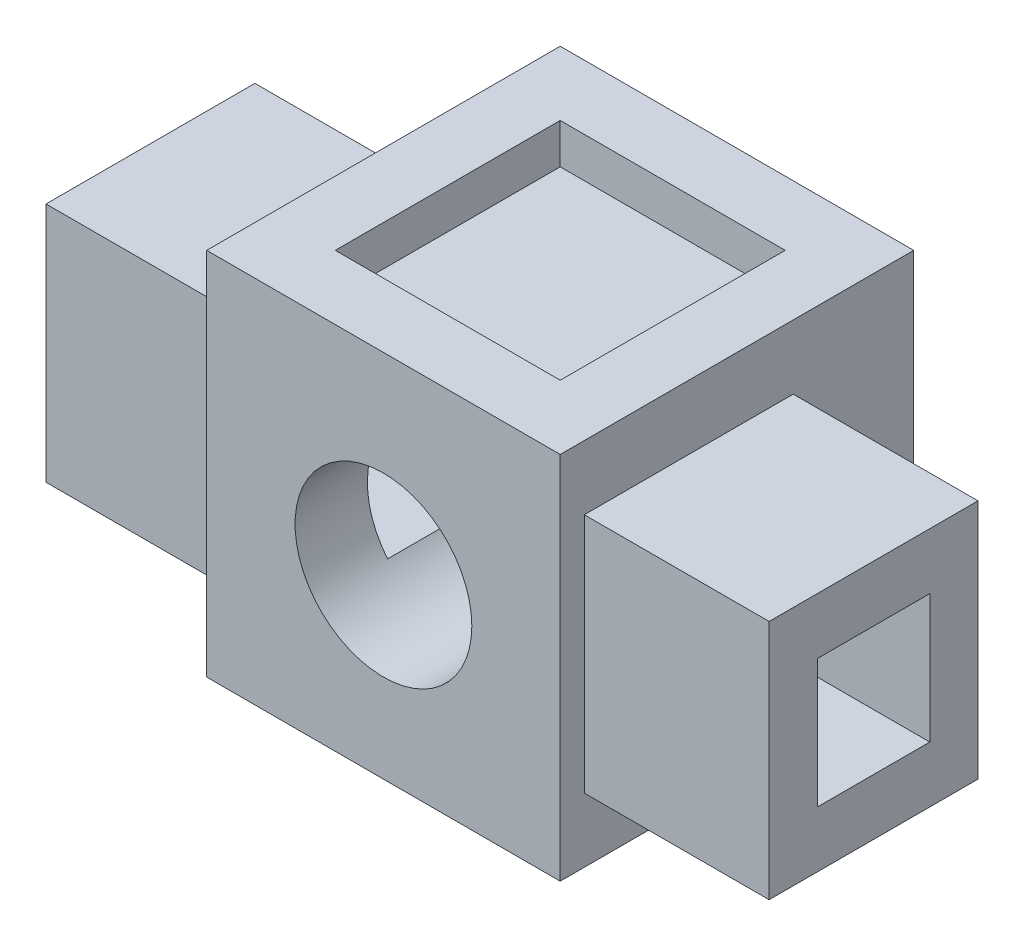
ISO-10303-21;
HEADER;
FILE_DESCRIPTION(('STEP AP214'),'2;1');
FILE_NAME('part.step','',(''),(''),'','','');
FILE_SCHEMA(('AUTOMOTIVE_DESIGN { 1 0 10303 214 1 1 1 1 }'));
ENDSEC;
DATA;
#1=APPLICATION_CONTEXT('core data for automotive mechanical design processes');
#2=APPLICATION_PROTOCOL_DEFINITION('international standard','automotive_design',2000,#1);
#3=PRODUCT_CONTEXT('',#1,'mechanical');
#4=PRODUCT('Part','Part','',(#3));
#5=PRODUCT_RELATED_PRODUCT_CATEGORY('part','',(#4));
#6=PRODUCT_DEFINITION_FORMATION('','',#4);
#7=PRODUCT_DEFINITION_CONTEXT('part definition',#1,'design');
#8=PRODUCT_DEFINITION('design','',#6,#7);
#9=PRODUCT_DEFINITION_SHAPE('','',#8);
#10=(LENGTH_UNIT() NAMED_UNIT(*) SI_UNIT(.MILLI.,.METRE.));
#11=(NAMED_UNIT(*) PLANE_ANGLE_UNIT() SI_UNIT($,.RADIAN.));
#12=(NAMED_UNIT(*) SI_UNIT($,.STERADIAN.) SOLID_ANGLE_UNIT());
#13=UNCERTAINTY_MEASURE_WITH_UNIT(LENGTH_MEASURE(1.E-05),#10,'distance_accuracy_value','');
#14=(GEOMETRIC_REPRESENTATION_CONTEXT(3) GLOBAL_UNCERTAINTY_ASSIGNED_CONTEXT((#13)) GLOBAL_UNIT_ASSIGNED_CONTEXT((#10,
#11,#12)) REPRESENTATION_CONTEXT('',''));
#15=CARTESIAN_POINT('',(0.,0.,0.));
#16=DIRECTION('',(0.,0.,1.));
#17=DIRECTION('',(1.,0.,0.));
#18=AXIS2_PLACEMENT_3D('',#15,#16,#17);
#19=CARTESIAN_POINT('',(22.,-23.,-44.));
#20=DIRECTION('',(1.,0.,0.));
#21=DIRECTION('',(0.,0.,-1.));
#22=AXIS2_PLACEMENT_3D('',#19,#20,#21);
#23=PLANE('',#22);
#24=DIRECTION('',(0.,1.,0.));
#25=VECTOR('',#24,1.);
#26=CARTESIAN_POINT('',(22.,-23.,0.));
#27=LINE('',#26,#25);
#28=CARTESIAN_POINT('',(22.,-23.,0.));
#29=VERTEX_POINT('',#28);
#30=CARTESIAN_POINT('',(22.,23.,0.));
#31=VERTEX_POINT('',#30);
#32=EDGE_CURVE('E360',#29,#31,#27,.T.);
#33=ORIENTED_EDGE('',*,*,#32,.F.);
#34=DIRECTION('',(0.,0.,1.));
#35=VECTOR('',#34,1.);
#36=CARTESIAN_POINT('',(22.,-23.,-44.));
#37=LINE('',#36,#35);
#38=CARTESIAN_POINT('',(22.,-23.,-44.));
#39=VERTEX_POINT('',#38);
#40=EDGE_CURVE('E11',#39,#29,#37,.T.);
#41=ORIENTED_EDGE('',*,*,#40,.F.);
#42=DIRECTION('',(0.,1.,0.));
#43=VECTOR('',#42,1.);
#44=CARTESIAN_POINT('',(22.,-23.,-44.));
#45=LINE('',#44,#43);
#46=CARTESIAN_POINT('',(22.,23.,-44.));
#47=VERTEX_POINT('',#46);
#48=EDGE_CURVE('E357',#39,#47,#45,.T.);
#49=ORIENTED_EDGE('',*,*,#48,.T.);
#50=DIRECTION('',(0.,0.,1.));
#51=VECTOR('',#50,1.);
#52=CARTESIAN_POINT('',(22.,23.,-44.));
#53=LINE('',#52,#51);
#54=EDGE_CURVE('E45',#47,#31,#53,.T.);
#55=ORIENTED_EDGE('',*,*,#54,.T.);
#56=EDGE_LOOP('',(#33,#41,#49,#55));
#57=FACE_BOUND('',#56,.T.);
#58=DIRECTION('',(0.,0.,1.));
#59=VECTOR('',#58,1.);
#60=CARTESIAN_POINT('',(22.,-15.,-29.));
#61=LINE('',#60,#59);
#62=CARTESIAN_POINT('',(22.,-15.,-29.));
#63=VERTEX_POINT('',#62);
#64=CARTESIAN_POINT('',(22.,-15.,-3.));
#65=VERTEX_POINT('',#64);
#66=EDGE_CURVE('E261',#63,#65,#61,.T.);
#67=ORIENTED_EDGE('',*,*,#66,.T.);
#68=DIRECTION('',(0.,1.,0.));
#69=VECTOR('',#68,1.);
#70=CARTESIAN_POINT('',(22.,15.,-3.));
#71=LINE('',#70,#69);
#72=CARTESIAN_POINT('',(22.,15.,-3.));
#73=VERTEX_POINT('',#72);
#74=EDGE_CURVE('E244',#65,#73,#71,.T.);
#75=ORIENTED_EDGE('',*,*,#74,.T.);
#76=DIRECTION('',(0.,0.,-1.));
#77=VECTOR('',#76,1.);
#78=CARTESIAN_POINT('',(22.,15.,-29.));
#79=LINE('',#78,#77);
#80=CARTESIAN_POINT('',(22.,15.,-29.));
#81=VERTEX_POINT('',#80);
#82=EDGE_CURVE('E249',#73,#81,#79,.T.);
#83=ORIENTED_EDGE('',*,*,#82,.T.);
#84=DIRECTION('',(0.,-1.,0.));
#85=VECTOR('',#84,1.);
#86=CARTESIAN_POINT('',(22.,15.,-29.));
#87=LINE('',#86,#85);
#88=EDGE_CURVE('E262',#81,#63,#87,.T.);
#89=ORIENTED_EDGE('',*,*,#88,.T.);
#90=EDGE_LOOP('',(#67,#75,#83,#89));
#91=FACE_BOUND('',#90,.T.);
#92=ADVANCED_FACE('F39',(#57,#91),#23,.T.);
#93=CARTESIAN_POINT('',(-22.,-23.,-44.));
#94=DIRECTION('',(-1.,0.,0.));
#95=DIRECTION('',(0.,0.,1.));
#96=AXIS2_PLACEMENT_3D('',#93,#94,#95);
#97=PLANE('',#96);
#98=DIRECTION('',(0.,-1.,0.));
#99=VECTOR('',#98,1.);
#100=CARTESIAN_POINT('',(-22.,-23.,0.));
#101=LINE('',#100,#99);
#102=CARTESIAN_POINT('',(-22.,23.,0.));
#103=VERTEX_POINT('',#102);
#104=CARTESIAN_POINT('',(-22.,-23.,0.));
#105=VERTEX_POINT('',#104);
#106=EDGE_CURVE('E378',#103,#105,#101,.T.);
#107=ORIENTED_EDGE('',*,*,#106,.F.);
#108=DIRECTION('',(0.,0.,1.));
#109=VECTOR('',#108,1.);
#110=CARTESIAN_POINT('',(-22.,23.,-44.));
#111=LINE('',#110,#109);
#112=CARTESIAN_POINT('',(-22.,23.,-44.));
#113=VERTEX_POINT('',#112);
#114=EDGE_CURVE('E382',#113,#103,#111,.T.);
#115=ORIENTED_EDGE('',*,*,#114,.F.);
#116=DIRECTION('',(0.,-1.,0.));
#117=VECTOR('',#116,1.);
#118=CARTESIAN_POINT('',(-22.,-23.,-44.));
#119=LINE('',#118,#117);
#120=CARTESIAN_POINT('',(-22.,-23.,-44.));
#121=VERTEX_POINT('',#120);
#122=EDGE_CURVE('E370',#113,#121,#119,.T.);
#123=ORIENTED_EDGE('',*,*,#122,.T.);
#124=DIRECTION('',(0.,0.,1.));
#125=VECTOR('',#124,1.);
#126=CARTESIAN_POINT('',(-22.,-23.,-44.));
#127=LINE('',#126,#125);
#128=EDGE_CURVE('E50',#121,#105,#127,.T.);
#129=ORIENTED_EDGE('',*,*,#128,.T.);
#130=EDGE_LOOP('',(#107,#115,#123,#129));
#131=FACE_BOUND('',#130,.T.);
#132=DIRECTION('',(0.,0.,-1.));
#133=VECTOR('',#132,1.);
#134=CARTESIAN_POINT('',(-22.,15.,-29.));
#135=LINE('',#134,#133);
#136=CARTESIAN_POINT('',(-22.,15.,-3.));
#137=VERTEX_POINT('',#136);
#138=CARTESIAN_POINT('',(-22.,15.,-29.));
#139=VERTEX_POINT('',#138);
#140=EDGE_CURVE('E308',#137,#139,#135,.T.);
#141=ORIENTED_EDGE('',*,*,#140,.F.);
#142=DIRECTION('',(0.,1.,0.));
#143=VECTOR('',#142,1.);
#144=CARTESIAN_POINT('',(-22.,15.,-3.));
#145=LINE('',#144,#143);
#146=CARTESIAN_POINT('',(-22.,-15.,-3.));
#147=VERTEX_POINT('',#146);
#148=EDGE_CURVE('E295',#147,#137,#145,.T.);
#149=ORIENTED_EDGE('',*,*,#148,.F.);
#150=DIRECTION('',(0.,0.,1.));
#151=VECTOR('',#150,1.);
#152=CARTESIAN_POINT('',(-22.,-15.,-29.));
#153=LINE('',#152,#151);
#154=CARTESIAN_POINT('',(-22.,-15.,-29.));
#155=VERTEX_POINT('',#154);
#156=EDGE_CURVE('E300',#155,#147,#153,.T.);
#157=ORIENTED_EDGE('',*,*,#156,.F.);
#158=DIRECTION('',(0.,-1.,0.));
#159=VECTOR('',#158,1.);
#160=CARTESIAN_POINT('',(-22.,15.,-29.));
#161=LINE('',#160,#159);
#162=EDGE_CURVE('E306',#139,#155,#161,.T.);
#163=ORIENTED_EDGE('',*,*,#162,.F.);
#164=EDGE_LOOP('',(#141,#149,#157,#163));
#165=FACE_BOUND('',#164,.T.);
#166=ADVANCED_FACE('F401',(#131,#165),#97,.T.);
#167=CARTESIAN_POINT('',(-22.,-23.,-44.));
#168=DIRECTION('',(0.,-1.,0.));
#169=DIRECTION('',(0.,0.,-1.));
#170=AXIS2_PLACEMENT_3D('',#167,#168,#169);
#171=PLANE('',#170);
#172=DIRECTION('',(1.,0.,0.));
#173=VECTOR('',#172,1.);
#174=CARTESIAN_POINT('',(-22.,-23.,0.));
#175=LINE('',#174,#173);
#176=EDGE_CURVE('E365',#105,#29,#175,.T.);
#177=ORIENTED_EDGE('',*,*,#176,.F.);
#178=ORIENTED_EDGE('',*,*,#128,.F.);
#179=DIRECTION('',(1.,0.,0.));
#180=VECTOR('',#179,1.);
#181=CARTESIAN_POINT('',(-22.,-23.,-44.));
#182=LINE('',#181,#180);
#183=EDGE_CURVE('E367',#121,#39,#182,.T.);
#184=ORIENTED_EDGE('',*,*,#183,.T.);
#185=ORIENTED_EDGE('',*,*,#40,.T.);
#186=EDGE_LOOP('',(#177,#178,#184,#185));
#187=FACE_BOUND('',#186,.T.);
#188=ADVANCED_FACE('F400',(#187),#171,.T.);
#189=CARTESIAN_POINT('',(-22.,23.,-44.));
#190=DIRECTION('',(0.,1.,0.));
#191=DIRECTION('',(0.,0.,1.));
#192=AXIS2_PLACEMENT_3D('',#189,#190,#191);
#193=PLANE('',#192);
#194=DIRECTION('',(0.,0.,-1.));
#195=VECTOR('',#194,1.);
#196=CARTESIAN_POINT('',(14.,23.,-8.));
#197=LINE('',#196,#195);
#198=CARTESIAN_POINT('',(14.,23.,-8.));
#199=VERTEX_POINT('',#198);
#200=CARTESIAN_POINT('',(14.,23.,-36.));
#201=VERTEX_POINT('',#200);
#202=EDGE_CURVE('E321',#199,#201,#197,.T.);
#203=ORIENTED_EDGE('',*,*,#202,.F.);
#204=DIRECTION('',(1.,0.,0.));
#205=VECTOR('',#204,1.);
#206=CARTESIAN_POINT('',(-14.,23.,-8.));
#207=LINE('',#206,#205);
#208=CARTESIAN_POINT('',(-14.,23.,-8.));
#209=VERTEX_POINT('',#208);
#210=EDGE_CURVE('E326',#209,#199,#207,.T.);
#211=ORIENTED_EDGE('',*,*,#210,.F.);
#212=DIRECTION('',(0.,0.,1.));
#213=VECTOR('',#212,1.);
#214=CARTESIAN_POINT('',(-14.,23.,-8.));
#215=LINE('',#214,#213);
#216=CARTESIAN_POINT('',(-14.,23.,-36.));
#217=VERTEX_POINT('',#216);
#218=EDGE_CURVE('E337',#217,#209,#215,.T.);
#219=ORIENTED_EDGE('',*,*,#218,.F.);
#220=DIRECTION('',(-1.,0.,0.));
#221=VECTOR('',#220,1.);
#222=CARTESIAN_POINT('',(-14.,23.,-36.));
#223=LINE('',#222,#221);
#224=EDGE_CURVE('E340',#201,#217,#223,.T.);
#225=ORIENTED_EDGE('',*,*,#224,.F.);
#226=EDGE_LOOP('',(#203,#211,#219,#225));
#227=FACE_BOUND('',#226,.T.);
#228=DIRECTION('',(-1.,0.,0.));
#229=VECTOR('',#228,1.);
#230=CARTESIAN_POINT('',(-22.,23.,0.));
#231=LINE('',#230,#229);
#232=EDGE_CURVE('E374',#31,#103,#231,.T.);
#233=ORIENTED_EDGE('',*,*,#232,.F.);
#234=ORIENTED_EDGE('',*,*,#54,.F.);
#235=DIRECTION('',(-1.,0.,0.));
#236=VECTOR('',#235,1.);
#237=CARTESIAN_POINT('',(-22.,23.,-44.));
#238=LINE('',#237,#236);
#239=EDGE_CURVE('E361',#47,#113,#238,.T.);
#240=ORIENTED_EDGE('',*,*,#239,.T.);
#241=ORIENTED_EDGE('',*,*,#114,.T.);
#242=EDGE_LOOP('',(#233,#234,#240,#241));
#243=FACE_BOUND('',#242,.T.);
#244=ADVANCED_FACE('F395',(#227,#243),#193,.T.);
#245=CARTESIAN_POINT('',(0.,0.,-44.));
#246=DIRECTION('',(0.,0.,-1.));
#247=DIRECTION('',(-1.,0.,0.));
#248=AXIS2_PLACEMENT_3D('',#245,#246,#247);
#249=PLANE('',#248);
#250=CARTESIAN_POINT('',(0.,-1.,-44.));
#251=DIRECTION('',(0.,0.,1.));
#252=DIRECTION('',(1.,0.,0.));
#253=AXIS2_PLACEMENT_3D('',#250,#251,#252);
#254=CIRCLE('',#253,11.);
#255=CARTESIAN_POINT('',(11.,-1.,-44.));
#256=VERTEX_POINT('',#255);
#257=EDGE_CURVE('E354',#256,#256,#254,.T.);
#258=ORIENTED_EDGE('',*,*,#257,.T.);
#259=EDGE_LOOP('',(#258));
#260=FACE_BOUND('',#259,.T.);
#261=ORIENTED_EDGE('',*,*,#48,.F.);
#262=ORIENTED_EDGE('',*,*,#183,.F.);
#263=ORIENTED_EDGE('',*,*,#122,.F.);
#264=ORIENTED_EDGE('',*,*,#239,.F.);
#265=EDGE_LOOP('',(#261,#262,#263,#264));
#266=FACE_BOUND('',#265,.T.);
#267=ADVANCED_FACE('F397',(#260,#266),#249,.T.);
#268=CARTESIAN_POINT('',(0.,0.,0.));
#269=DIRECTION('',(0.,0.,-1.));
#270=DIRECTION('',(-1.,0.,0.));
#271=AXIS2_PLACEMENT_3D('',#268,#269,#270);
#272=PLANE('',#271);
#273=CARTESIAN_POINT('',(0.,-1.,0.));
#274=DIRECTION('',(0.,0.,1.));
#275=DIRECTION('',(1.,0.,0.));
#276=AXIS2_PLACEMENT_3D('',#273,#274,#275);
#277=CIRCLE('',#276,11.);
#278=CARTESIAN_POINT('',(11.,-1.,0.));
#279=VERTEX_POINT('',#278);
#280=EDGE_CURVE('E350',#279,#279,#277,.T.);
#281=ORIENTED_EDGE('',*,*,#280,.F.);
#282=EDGE_LOOP('',(#281));
#283=FACE_BOUND('',#282,.T.);
#284=ORIENTED_EDGE('',*,*,#32,.T.);
#285=ORIENTED_EDGE('',*,*,#232,.T.);
#286=ORIENTED_EDGE('',*,*,#106,.T.);
#287=ORIENTED_EDGE('',*,*,#176,.T.);
#288=EDGE_LOOP('',(#284,#285,#286,#287));
#289=FACE_BOUND('',#288,.T.);
#290=ADVANCED_FACE('F394',(#283,#289),#272,.F.);
#291=CARTESIAN_POINT('',(0.,-1.,-44.));
#292=DIRECTION('',(0.,0.,1.));
#293=DIRECTION('',(1.,0.,0.));
#294=AXIS2_PLACEMENT_3D('',#291,#292,#293);
#295=CYLINDRICAL_SURFACE('',#294,11.);
#296=CARTESIAN_POINT('',(0.,-1.,-8.99999999999999));
#297=DIRECTION('',(0.,0.,1.));
#298=DIRECTION('',(0.,-1.,0.));
#299=AXIS2_PLACEMENT_3D('',#296,#297,#298);
#300=CIRCLE('',#299,11.);
#301=CARTESIAN_POINT('',(6.32455532033675,8.,-9.));
#302=VERTEX_POINT('',#301);
#303=CARTESIAN_POINT('',(8.48528137423857,-8.,-8.99999999999999));
#304=VERTEX_POINT('',#303);
#305=EDGE_CURVE('E224',#302,#304,#300,.F.);
#306=ORIENTED_EDGE('',*,*,#305,.T.);
#307=DIRECTION('',(0.,0.,1.));
#308=VECTOR('',#307,1.);
#309=CARTESIAN_POINT('',(8.48528137423857,-8.,-44.));
#310=LINE('',#309,#308);
#311=CARTESIAN_POINT('',(8.48528137423857,-8.,-23.));
#312=VERTEX_POINT('',#311);
#313=EDGE_CURVE('E202',#304,#312,#310,.F.);
#314=ORIENTED_EDGE('',*,*,#313,.T.);
#315=CARTESIAN_POINT('',(0.,-1.,-23.));
#316=DIRECTION('',(0.,0.,-1.));
#317=DIRECTION('',(-1.,0.,0.));
#318=AXIS2_PLACEMENT_3D('',#315,#316,#317);
#319=CIRCLE('',#318,11.);
#320=CARTESIAN_POINT('',(6.32455532033676,8.,-23.));
#321=VERTEX_POINT('',#320);
#322=EDGE_CURVE('E213',#312,#321,#319,.F.);
#323=ORIENTED_EDGE('',*,*,#322,.T.);
#324=DIRECTION('',(0.,0.,1.));
#325=VECTOR('',#324,1.);
#326=CARTESIAN_POINT('',(6.32455532033676,8.,-44.));
#327=LINE('',#326,#325);
#328=EDGE_CURVE('E220',#321,#302,#327,.T.);
#329=ORIENTED_EDGE('',*,*,#328,.T.);
#330=EDGE_LOOP('',(#306,#314,#323,#329));
#331=FACE_BOUND('',#330,.T.);
#332=CARTESIAN_POINT('',(-6.32455532033676,8.,-23.));
#333=VERTEX_POINT('',#332);
#334=CARTESIAN_POINT('',(-8.48528137423857,-8.,-23.));
#335=VERTEX_POINT('',#334);
#336=EDGE_CURVE('E217',#333,#335,#319,.F.);
#337=ORIENTED_EDGE('',*,*,#336,.T.);
#338=DIRECTION('',(0.,0.,1.));
#339=VECTOR('',#338,1.);
#340=CARTESIAN_POINT('',(-8.48528137423857,-8.,-44.));
#341=LINE('',#340,#339);
#342=CARTESIAN_POINT('',(-8.48528137423857,-8.,-8.99999999999999));
#343=VERTEX_POINT('',#342);
#344=EDGE_CURVE('E223',#335,#343,#341,.T.);
#345=ORIENTED_EDGE('',*,*,#344,.T.);
#346=CARTESIAN_POINT('',(-6.32455532033677,8.,-9.));
#347=VERTEX_POINT('',#346);
#348=EDGE_CURVE('E227',#343,#347,#300,.F.);
#349=ORIENTED_EDGE('',*,*,#348,.T.);
#350=DIRECTION('',(0.,0.,1.));
#351=VECTOR('',#350,1.);
#352=CARTESIAN_POINT('',(-6.32455532033676,8.,-44.));
#353=LINE('',#352,#351);
#354=EDGE_CURVE('E740',#347,#333,#353,.F.);
#355=ORIENTED_EDGE('',*,*,#354,.T.);
#356=EDGE_LOOP('',(#337,#345,#349,#355));
#357=FACE_BOUND('',#356,.T.);
#358=ORIENTED_EDGE('',*,*,#257,.F.);
#359=EDGE_LOOP('',(#358));
#360=FACE_BOUND('',#359,.T.);
#361=ORIENTED_EDGE('',*,*,#280,.T.);
#362=EDGE_LOOP('',(#361));
#363=FACE_BOUND('',#362,.T.);
#364=ADVANCED_FACE('F219',(#331,#357,#360,#363),#295,.F.);
#365=CARTESIAN_POINT('',(14.,18.,-8.));
#366=DIRECTION('',(1.,0.,0.));
#367=DIRECTION('',(0.,0.,-1.));
#368=AXIS2_PLACEMENT_3D('',#365,#366,#367);
#369=PLANE('',#368);
#370=ORIENTED_EDGE('',*,*,#202,.T.);
#371=DIRECTION('',(0.,1.,0.));
#372=VECTOR('',#371,1.);
#373=CARTESIAN_POINT('',(14.,18.,-36.));
#374=LINE('',#373,#372);
#375=CARTESIAN_POINT('',(14.,18.,-36.));
#376=VERTEX_POINT('',#375);
#377=EDGE_CURVE('E333',#376,#201,#374,.T.);
#378=ORIENTED_EDGE('',*,*,#377,.F.);
#379=DIRECTION('',(0.,0.,-1.));
#380=VECTOR('',#379,1.);
#381=CARTESIAN_POINT('',(14.,18.,-8.));
#382=LINE('',#381,#380);
#383=CARTESIAN_POINT('',(14.,18.,-8.));
#384=VERTEX_POINT('',#383);
#385=EDGE_CURVE('E325',#384,#376,#382,.T.);
#386=ORIENTED_EDGE('',*,*,#385,.F.);
#387=DIRECTION('',(0.,1.,0.));
#388=VECTOR('',#387,1.);
#389=CARTESIAN_POINT('',(14.,18.,-8.));
#390=LINE('',#389,#388);
#391=EDGE_CURVE('E342',#384,#199,#390,.T.);
#392=ORIENTED_EDGE('',*,*,#391,.T.);
#393=EDGE_LOOP('',(#370,#378,#386,#392));
#394=FACE_BOUND('',#393,.T.);
#395=ADVANCED_FACE('F499',(#394),#369,.F.);
#396=CARTESIAN_POINT('',(-14.,18.,-8.));
#397=DIRECTION('',(0.,0.,1.));
#398=DIRECTION('',(1.,0.,0.));
#399=AXIS2_PLACEMENT_3D('',#396,#397,#398);
#400=PLANE('',#399);
#401=ORIENTED_EDGE('',*,*,#210,.T.);
#402=ORIENTED_EDGE('',*,*,#391,.F.);
#403=DIRECTION('',(1.,0.,0.));
#404=VECTOR('',#403,1.);
#405=CARTESIAN_POINT('',(-14.,18.,-8.));
#406=LINE('',#405,#404);
#407=CARTESIAN_POINT('',(-14.,18.,-8.));
#408=VERTEX_POINT('',#407);
#409=EDGE_CURVE('E335',#408,#384,#406,.T.);
#410=ORIENTED_EDGE('',*,*,#409,.F.);
#411=DIRECTION('',(0.,1.,0.));
#412=VECTOR('',#411,1.);
#413=CARTESIAN_POINT('',(-14.,18.,-8.));
#414=LINE('',#413,#412);
#415=EDGE_CURVE('E346',#408,#209,#414,.T.);
#416=ORIENTED_EDGE('',*,*,#415,.T.);
#417=EDGE_LOOP('',(#401,#402,#410,#416));
#418=FACE_BOUND('',#417,.T.);
#419=ADVANCED_FACE('F602',(#418),#400,.F.);
#420=CARTESIAN_POINT('',(-14.,18.,-8.));
#421=DIRECTION('',(-1.,0.,0.));
#422=DIRECTION('',(0.,0.,1.));
#423=AXIS2_PLACEMENT_3D('',#420,#421,#422);
#424=PLANE('',#423);
#425=ORIENTED_EDGE('',*,*,#218,.T.);
#426=ORIENTED_EDGE('',*,*,#415,.F.);
#427=DIRECTION('',(0.,0.,1.));
#428=VECTOR('',#427,1.);
#429=CARTESIAN_POINT('',(-14.,18.,-8.));
#430=LINE('',#429,#428);
#431=CARTESIAN_POINT('',(-14.,18.,-36.));
#432=VERTEX_POINT('',#431);
#433=EDGE_CURVE('E328',#432,#408,#430,.T.);
#434=ORIENTED_EDGE('',*,*,#433,.F.);
#435=DIRECTION('',(0.,1.,0.));
#436=VECTOR('',#435,1.);
#437=CARTESIAN_POINT('',(-14.,18.,-36.));
#438=LINE('',#437,#436);
#439=EDGE_CURVE('E348',#432,#217,#438,.T.);
#440=ORIENTED_EDGE('',*,*,#439,.T.);
#441=EDGE_LOOP('',(#425,#426,#434,#440));
#442=FACE_BOUND('',#441,.T.);
#443=ADVANCED_FACE('F598',(#442),#424,.F.);
#444=CARTESIAN_POINT('',(-14.,18.,-36.));
#445=DIRECTION('',(0.,0.,-1.));
#446=DIRECTION('',(-1.,0.,0.));
#447=AXIS2_PLACEMENT_3D('',#444,#445,#446);
#448=PLANE('',#447);
#449=ORIENTED_EDGE('',*,*,#224,.T.);
#450=ORIENTED_EDGE('',*,*,#439,.F.);
#451=DIRECTION('',(-1.,0.,0.));
#452=VECTOR('',#451,1.);
#453=CARTESIAN_POINT('',(-14.,18.,-36.));
#454=LINE('',#453,#452);
#455=EDGE_CURVE('E324',#376,#432,#454,.T.);
#456=ORIENTED_EDGE('',*,*,#455,.F.);
#457=ORIENTED_EDGE('',*,*,#377,.T.);
#458=EDGE_LOOP('',(#449,#450,#456,#457));
#459=FACE_BOUND('',#458,.T.);
#460=ADVANCED_FACE('F595',(#459),#448,.F.);
#461=CARTESIAN_POINT('',(0.,18.,0.));
#462=DIRECTION('',(0.,-1.,0.));
#463=DIRECTION('',(0.,0.,-1.));
#464=AXIS2_PLACEMENT_3D('',#461,#462,#463);
#465=PLANE('',#464);
#466=ORIENTED_EDGE('',*,*,#385,.T.);
#467=ORIENTED_EDGE('',*,*,#455,.T.);
#468=ORIENTED_EDGE('',*,*,#433,.T.);
#469=ORIENTED_EDGE('',*,*,#409,.T.);
#470=EDGE_LOOP('',(#466,#467,#468,#469));
#471=FACE_BOUND('',#470,.T.);
#472=ADVANCED_FACE('F588',(#471),#465,.F.);
#473=CARTESIAN_POINT('',(-45.,0.,0.));
#474=DIRECTION('',(-1.,0.,0.));
#475=DIRECTION('',(0.,0.,1.));
#476=AXIS2_PLACEMENT_3D('',#473,#474,#475);
#477=PLANE('',#476);
#478=DIRECTION('',(0.,1.,0.));
#479=VECTOR('',#478,1.);
#480=CARTESIAN_POINT('',(-45.,15.,-3.));
#481=LINE('',#480,#479);
#482=CARTESIAN_POINT('',(-45.,-15.,-3.));
#483=VERTEX_POINT('',#482);
#484=CARTESIAN_POINT('',(-45.,15.,-3.));
#485=VERTEX_POINT('',#484);
#486=EDGE_CURVE('E291',#483,#485,#481,.T.);
#487=ORIENTED_EDGE('',*,*,#486,.T.);
#488=DIRECTION('',(0.,0.,-1.));
#489=VECTOR('',#488,1.);
#490=CARTESIAN_POINT('',(-45.,15.,-29.));
#491=LINE('',#490,#489);
#492=CARTESIAN_POINT('',(-45.,15.,-29.));
#493=VERTEX_POINT('',#492);
#494=EDGE_CURVE('E298',#485,#493,#491,.T.);
#495=ORIENTED_EDGE('',*,*,#494,.T.);
#496=DIRECTION('',(0.,-1.,0.));
#497=VECTOR('',#496,1.);
#498=CARTESIAN_POINT('',(-45.,15.,-29.));
#499=LINE('',#498,#497);
#500=CARTESIAN_POINT('',(-45.,-15.,-29.));
#501=VERTEX_POINT('',#500);
#502=EDGE_CURVE('E299',#493,#501,#499,.T.);
#503=ORIENTED_EDGE('',*,*,#502,.T.);
#504=DIRECTION('',(0.,0.,1.));
#505=VECTOR('',#504,1.);
#506=CARTESIAN_POINT('',(-45.,-15.,-29.));
#507=LINE('',#506,#505);
#508=EDGE_CURVE('E303',#501,#483,#507,.T.);
#509=ORIENTED_EDGE('',*,*,#508,.T.);
#510=EDGE_LOOP('',(#487,#495,#503,#509));
#511=FACE_BOUND('',#510,.T.);
#512=DIRECTION('',(0.,0.,-1.));
#513=VECTOR('',#512,1.);
#514=CARTESIAN_POINT('',(-45.,8.,-23.));
#515=LINE('',#514,#513);
#516=CARTESIAN_POINT('',(-45.,8.,-9.));
#517=VERTEX_POINT('',#516);
#518=CARTESIAN_POINT('',(-45.,8.,-23.));
#519=VERTEX_POINT('',#518);
#520=EDGE_CURVE('E276',#517,#519,#515,.T.);
#521=ORIENTED_EDGE('',*,*,#520,.F.);
#522=DIRECTION('',(0.,1.,0.));
#523=VECTOR('',#522,1.);
#524=CARTESIAN_POINT('',(-45.,8.,-9.));
#525=LINE('',#524,#523);
#526=CARTESIAN_POINT('',(-45.,-8.,-9.));
#527=VERTEX_POINT('',#526);
#528=EDGE_CURVE('E280',#527,#517,#525,.T.);
#529=ORIENTED_EDGE('',*,*,#528,.F.);
#530=DIRECTION('',(0.,0.,1.));
#531=VECTOR('',#530,1.);
#532=CARTESIAN_POINT('',(-45.,-8.,-23.));
#533=LINE('',#532,#531);
#534=CARTESIAN_POINT('',(-45.,-8.,-23.));
#535=VERTEX_POINT('',#534);
#536=EDGE_CURVE('E281',#535,#527,#533,.T.);
#537=ORIENTED_EDGE('',*,*,#536,.F.);
#538=DIRECTION('',(0.,-1.,0.));
#539=VECTOR('',#538,1.);
#540=CARTESIAN_POINT('',(-45.,8.,-23.));
#541=LINE('',#540,#539);
#542=EDGE_CURVE('E283',#519,#535,#541,.T.);
#543=ORIENTED_EDGE('',*,*,#542,.F.);
#544=EDGE_LOOP('',(#521,#529,#537,#543));
#545=FACE_BOUND('',#544,.T.);
#546=ADVANCED_FACE('F423',(#511,#545),#477,.T.);
#547=CARTESIAN_POINT('',(-45.,15.,-3.));
#548=DIRECTION('',(0.,0.,-1.));
#549=DIRECTION('',(0.,1.,0.));
#550=AXIS2_PLACEMENT_3D('',#547,#548,#549);
#551=PLANE('',#550);
#552=ORIENTED_EDGE('',*,*,#148,.T.);
#553=DIRECTION('',(1.,0.,0.));
#554=VECTOR('',#553,1.);
#555=CARTESIAN_POINT('',(-45.,15.,-3.));
#556=LINE('',#555,#554);
#557=EDGE_CURVE('E317',#485,#137,#556,.T.);
#558=ORIENTED_EDGE('',*,*,#557,.F.);
#559=ORIENTED_EDGE('',*,*,#486,.F.);
#560=DIRECTION('',(1.,0.,0.));
#561=VECTOR('',#560,1.);
#562=CARTESIAN_POINT('',(-45.,-15.,-3.));
#563=LINE('',#562,#561);
#564=EDGE_CURVE('E301',#483,#147,#563,.T.);
#565=ORIENTED_EDGE('',*,*,#564,.T.);
#566=EDGE_LOOP('',(#552,#558,#559,#565));
#567=FACE_BOUND('',#566,.T.);
#568=ADVANCED_FACE('F426',(#567),#551,.F.);
#569=CARTESIAN_POINT('',(-45.,15.,-29.));
#570=DIRECTION('',(0.,-1.,0.));
#571=DIRECTION('',(0.,0.,-1.));
#572=AXIS2_PLACEMENT_3D('',#569,#570,#571);
#573=PLANE('',#572);
#574=ORIENTED_EDGE('',*,*,#140,.T.);
#575=DIRECTION('',(1.,0.,0.));
#576=VECTOR('',#575,1.);
#577=CARTESIAN_POINT('',(-45.,15.,-29.));
#578=LINE('',#577,#576);
#579=EDGE_CURVE('E316',#493,#139,#578,.T.);
#580=ORIENTED_EDGE('',*,*,#579,.F.);
#581=ORIENTED_EDGE('',*,*,#494,.F.);
#582=ORIENTED_EDGE('',*,*,#557,.T.);
#583=EDGE_LOOP('',(#574,#580,#581,#582));
#584=FACE_BOUND('',#583,.T.);
#585=ADVANCED_FACE('F411',(#584),#573,.F.);
#586=CARTESIAN_POINT('',(-45.,15.,-29.));
#587=DIRECTION('',(0.,0.,1.));
#588=DIRECTION('',(0.,-1.,0.));
#589=AXIS2_PLACEMENT_3D('',#586,#587,#588);
#590=PLANE('',#589);
#591=ORIENTED_EDGE('',*,*,#162,.T.);
#592=DIRECTION('',(1.,0.,0.));
#593=VECTOR('',#592,1.);
#594=CARTESIAN_POINT('',(-45.,-15.,-29.));
#595=LINE('',#594,#593);
#596=EDGE_CURVE('E314',#501,#155,#595,.T.);
#597=ORIENTED_EDGE('',*,*,#596,.F.);
#598=ORIENTED_EDGE('',*,*,#502,.F.);
#599=ORIENTED_EDGE('',*,*,#579,.T.);
#600=EDGE_LOOP('',(#591,#597,#598,#599));
#601=FACE_BOUND('',#600,.T.);
#602=ADVANCED_FACE('F417',(#601),#590,.F.);
#603=CARTESIAN_POINT('',(-45.,-15.,-29.));
#604=DIRECTION('',(0.,1.,0.));
#605=DIRECTION('',(0.,0.,1.));
#606=AXIS2_PLACEMENT_3D('',#603,#604,#605);
#607=PLANE('',#606);
#608=ORIENTED_EDGE('',*,*,#156,.T.);
#609=ORIENTED_EDGE('',*,*,#564,.F.);
#610=ORIENTED_EDGE('',*,*,#508,.F.);
#611=ORIENTED_EDGE('',*,*,#596,.T.);
#612=EDGE_LOOP('',(#608,#609,#610,#611));
#613=FACE_BOUND('',#612,.T.);
#614=ADVANCED_FACE('F428',(#613),#607,.F.);
#615=CARTESIAN_POINT('',(-45.,8.,-9.));
#616=DIRECTION('',(0.,0.,-1.));
#617=DIRECTION('',(0.,1.,0.));
#618=AXIS2_PLACEMENT_3D('',#615,#616,#617);
#619=PLANE('',#618);
#620=DIRECTION('',(1.,0.,0.));
#621=VECTOR('',#620,1.);
#622=CARTESIAN_POINT('',(-45.,8.,-9.));
#623=LINE('',#622,#621);
#624=EDGE_CURVE('E287',#517,#347,#623,.T.);
#625=ORIENTED_EDGE('',*,*,#624,.T.);
#626=ORIENTED_EDGE('',*,*,#348,.F.);
#627=DIRECTION('',(1.,0.,0.));
#628=VECTOR('',#627,1.);
#629=CARTESIAN_POINT('',(-45.,-8.,-9.));
#630=LINE('',#629,#628);
#631=EDGE_CURVE('E282',#527,#343,#630,.T.);
#632=ORIENTED_EDGE('',*,*,#631,.F.);
#633=ORIENTED_EDGE('',*,*,#528,.T.);
#634=EDGE_LOOP('',(#625,#626,#632,#633));
#635=FACE_BOUND('',#634,.T.);
#636=ADVANCED_FACE('F429',(#635),#619,.T.);
#637=CARTESIAN_POINT('',(-45.,8.,-23.));
#638=DIRECTION('',(0.,-1.,0.));
#639=DIRECTION('',(0.,0.,-1.));
#640=AXIS2_PLACEMENT_3D('',#637,#638,#639);
#641=PLANE('',#640);
#642=DIRECTION('',(1.,0.,0.));
#643=VECTOR('',#642,1.);
#644=CARTESIAN_POINT('',(-45.,8.,-23.));
#645=LINE('',#644,#643);
#646=EDGE_CURVE('E286',#519,#333,#645,.T.);
#647=ORIENTED_EDGE('',*,*,#646,.T.);
#648=ORIENTED_EDGE('',*,*,#354,.F.);
#649=ORIENTED_EDGE('',*,*,#624,.F.);
#650=ORIENTED_EDGE('',*,*,#520,.T.);
#651=EDGE_LOOP('',(#647,#648,#649,#650));
#652=FACE_BOUND('',#651,.T.);
#653=ADVANCED_FACE('F440',(#652),#641,.T.);
#654=CARTESIAN_POINT('',(-45.,8.,-23.));
#655=DIRECTION('',(0.,0.,1.));
#656=DIRECTION('',(1.,0.,0.));
#657=AXIS2_PLACEMENT_3D('',#654,#655,#656);
#658=PLANE('',#657);
#659=DIRECTION('',(1.,0.,0.));
#660=VECTOR('',#659,1.);
#661=CARTESIAN_POINT('',(-45.,-8.,-23.));
#662=LINE('',#661,#660);
#663=EDGE_CURVE('E61',#535,#335,#662,.T.);
#664=ORIENTED_EDGE('',*,*,#663,.T.);
#665=ORIENTED_EDGE('',*,*,#336,.F.);
#666=ORIENTED_EDGE('',*,*,#646,.F.);
#667=ORIENTED_EDGE('',*,*,#542,.T.);
#668=EDGE_LOOP('',(#664,#665,#666,#667));
#669=FACE_BOUND('',#668,.T.);
#670=ADVANCED_FACE('F513',(#669),#658,.T.);
#671=CARTESIAN_POINT('',(-45.,-8.,-23.));
#672=DIRECTION('',(0.,1.,0.));
#673=DIRECTION('',(0.,0.,1.));
#674=AXIS2_PLACEMENT_3D('',#671,#672,#673);
#675=PLANE('',#674);
#676=ORIENTED_EDGE('',*,*,#631,.T.);
#677=ORIENTED_EDGE('',*,*,#344,.F.);
#678=ORIENTED_EDGE('',*,*,#663,.F.);
#679=ORIENTED_EDGE('',*,*,#536,.T.);
#680=EDGE_LOOP('',(#676,#677,#678,#679));
#681=FACE_BOUND('',#680,.T.);
#682=ADVANCED_FACE('F454',(#681),#675,.T.);
#683=CARTESIAN_POINT('',(45.,15.,-3.));
#684=DIRECTION('',(0.,0.,1.));
#685=DIRECTION('',(0.,-1.,0.));
#686=AXIS2_PLACEMENT_3D('',#683,#684,#685);
#687=PLANE('',#686);
#688=ORIENTED_EDGE('',*,*,#74,.F.);
#689=DIRECTION('',(-1.,0.,0.));
#690=VECTOR('',#689,1.);
#691=CARTESIAN_POINT('',(45.,-15.,-3.));
#692=LINE('',#691,#690);
#693=CARTESIAN_POINT('',(45.,-15.,-3.));
#694=VERTEX_POINT('',#693);
#695=EDGE_CURVE('E273',#694,#65,#692,.T.);
#696=ORIENTED_EDGE('',*,*,#695,.F.);
#697=DIRECTION('',(0.,1.,0.));
#698=VECTOR('',#697,1.);
#699=CARTESIAN_POINT('',(45.,15.,-3.));
#700=LINE('',#699,#698);
#701=CARTESIAN_POINT('',(45.,15.,-3.));
#702=VERTEX_POINT('',#701);
#703=EDGE_CURVE('E242',#694,#702,#700,.T.);
#704=ORIENTED_EDGE('',*,*,#703,.T.);
#705=DIRECTION('',(-1.,0.,0.));
#706=VECTOR('',#705,1.);
#707=CARTESIAN_POINT('',(45.,15.,-3.));
#708=LINE('',#707,#706);
#709=EDGE_CURVE('E256',#702,#73,#708,.T.);
#710=ORIENTED_EDGE('',*,*,#709,.T.);
#711=EDGE_LOOP('',(#688,#696,#704,#710));
#712=FACE_BOUND('',#711,.T.);
#713=ADVANCED_FACE('F449',(#712),#687,.T.);
#714=CARTESIAN_POINT('',(45.,-15.,-29.));
#715=DIRECTION('',(0.,-1.,0.));
#716=DIRECTION('',(0.,0.,-1.));
#717=AXIS2_PLACEMENT_3D('',#714,#715,#716);
#718=PLANE('',#717);
#719=ORIENTED_EDGE('',*,*,#66,.F.);
#720=DIRECTION('',(-1.,0.,0.));
#721=VECTOR('',#720,1.);
#722=CARTESIAN_POINT('',(45.,-15.,-29.));
#723=LINE('',#722,#721);
#724=CARTESIAN_POINT('',(45.,-15.,-29.));
#725=VERTEX_POINT('',#724);
#726=EDGE_CURVE('E275',#725,#63,#723,.T.);
#727=ORIENTED_EDGE('',*,*,#726,.F.);
#728=DIRECTION('',(0.,0.,1.));
#729=VECTOR('',#728,1.);
#730=CARTESIAN_POINT('',(45.,-15.,-29.));
#731=LINE('',#730,#729);
#732=EDGE_CURVE('E246',#725,#694,#731,.T.);
#733=ORIENTED_EDGE('',*,*,#732,.T.);
#734=ORIENTED_EDGE('',*,*,#695,.T.);
#735=EDGE_LOOP('',(#719,#727,#733,#734));
#736=FACE_BOUND('',#735,.T.);
#737=ADVANCED_FACE('F451',(#736),#718,.T.);
#738=CARTESIAN_POINT('',(45.,15.,-29.));
#739=DIRECTION('',(0.,0.,-1.));
#740=DIRECTION('',(0.,1.,0.));
#741=AXIS2_PLACEMENT_3D('',#738,#739,#740);
#742=PLANE('',#741);
#743=ORIENTED_EDGE('',*,*,#88,.F.);
#744=DIRECTION('',(-1.,0.,0.));
#745=VECTOR('',#744,1.);
#746=CARTESIAN_POINT('',(45.,15.,-29.));
#747=LINE('',#746,#745);
#748=CARTESIAN_POINT('',(45.,15.,-29.));
#749=VERTEX_POINT('',#748);
#750=EDGE_CURVE('E269',#749,#81,#747,.T.);
#751=ORIENTED_EDGE('',*,*,#750,.F.);
#752=DIRECTION('',(0.,-1.,0.));
#753=VECTOR('',#752,1.);
#754=CARTESIAN_POINT('',(45.,15.,-29.));
#755=LINE('',#754,#753);
#756=EDGE_CURVE('E252',#749,#725,#755,.T.);
#757=ORIENTED_EDGE('',*,*,#756,.T.);
#758=ORIENTED_EDGE('',*,*,#726,.T.);
#759=EDGE_LOOP('',(#743,#751,#757,#758));
#760=FACE_BOUND('',#759,.T.);
#761=ADVANCED_FACE('F465',(#760),#742,.T.);
#762=CARTESIAN_POINT('',(45.,15.,-29.));
#763=DIRECTION('',(0.,1.,0.));
#764=DIRECTION('',(0.,0.,1.));
#765=AXIS2_PLACEMENT_3D('',#762,#763,#764);
#766=PLANE('',#765);
#767=ORIENTED_EDGE('',*,*,#82,.F.);
#768=ORIENTED_EDGE('',*,*,#709,.F.);
#769=DIRECTION('',(0.,0.,-1.));
#770=VECTOR('',#769,1.);
#771=CARTESIAN_POINT('',(45.,15.,-29.));
#772=LINE('',#771,#770);
#773=EDGE_CURVE('E254',#702,#749,#772,.T.);
#774=ORIENTED_EDGE('',*,*,#773,.T.);
#775=ORIENTED_EDGE('',*,*,#750,.T.);
#776=EDGE_LOOP('',(#767,#768,#774,#775));
#777=FACE_BOUND('',#776,.T.);
#778=ADVANCED_FACE('F473',(#777),#766,.T.);
#779=CARTESIAN_POINT('',(45.,0.,0.));
#780=DIRECTION('',(1.,0.,0.));
#781=DIRECTION('',(0.,0.,1.));
#782=AXIS2_PLACEMENT_3D('',#779,#780,#781);
#783=PLANE('',#782);
#784=DIRECTION('',(0.,1.,0.));
#785=VECTOR('',#784,1.);
#786=CARTESIAN_POINT('',(45.,8.,-9.));
#787=LINE('',#786,#785);
#788=CARTESIAN_POINT('',(45.,-8.,-9.));
#789=VERTEX_POINT('',#788);
#790=CARTESIAN_POINT('',(45.,8.,-9.));
#791=VERTEX_POINT('',#790);
#792=EDGE_CURVE('E221',#789,#791,#787,.T.);
#793=ORIENTED_EDGE('',*,*,#792,.T.);
#794=DIRECTION('',(0.,0.,-1.));
#795=VECTOR('',#794,1.);
#796=CARTESIAN_POINT('',(45.,8.,-23.));
#797=LINE('',#796,#795);
#798=CARTESIAN_POINT('',(45.,8.,-23.));
#799=VERTEX_POINT('',#798);
#800=EDGE_CURVE('E240',#791,#799,#797,.T.);
#801=ORIENTED_EDGE('',*,*,#800,.T.);
#802=DIRECTION('',(0.,-1.,0.));
#803=VECTOR('',#802,1.);
#804=CARTESIAN_POINT('',(45.,8.,-23.));
#805=LINE('',#804,#803);
#806=CARTESIAN_POINT('',(45.,-8.,-23.));
#807=VERTEX_POINT('',#806);
#808=EDGE_CURVE('E232',#799,#807,#805,.T.);
#809=ORIENTED_EDGE('',*,*,#808,.T.);
#810=DIRECTION('',(0.,0.,1.));
#811=VECTOR('',#810,1.);
#812=CARTESIAN_POINT('',(45.,-8.,-23.));
#813=LINE('',#812,#811);
#814=EDGE_CURVE('E208',#807,#789,#813,.T.);
#815=ORIENTED_EDGE('',*,*,#814,.T.);
#816=EDGE_LOOP('',(#793,#801,#809,#815));
#817=FACE_BOUND('',#816,.T.);
#818=ORIENTED_EDGE('',*,*,#703,.F.);
#819=ORIENTED_EDGE('',*,*,#732,.F.);
#820=ORIENTED_EDGE('',*,*,#756,.F.);
#821=ORIENTED_EDGE('',*,*,#773,.F.);
#822=EDGE_LOOP('',(#818,#819,#820,#821));
#823=FACE_BOUND('',#822,.T.);
#824=ADVANCED_FACE('F477',(#817,#823),#783,.T.);
#825=CARTESIAN_POINT('',(45.,8.,-9.));
#826=DIRECTION('',(0.,0.,1.));
#827=DIRECTION('',(0.,-1.,0.));
#828=AXIS2_PLACEMENT_3D('',#825,#826,#827);
#829=PLANE('',#828);
#830=DIRECTION('',(-1.,0.,0.));
#831=VECTOR('',#830,1.);
#832=CARTESIAN_POINT('',(45.,-8.,-9.));
#833=LINE('',#832,#831);
#834=EDGE_CURVE('E209',#789,#304,#833,.T.);
#835=ORIENTED_EDGE('',*,*,#834,.T.);
#836=ORIENTED_EDGE('',*,*,#305,.F.);
#837=DIRECTION('',(-1.,0.,0.));
#838=VECTOR('',#837,1.);
#839=CARTESIAN_POINT('',(45.,8.,-9.));
#840=LINE('',#839,#838);
#841=EDGE_CURVE('E238',#791,#302,#840,.T.);
#842=ORIENTED_EDGE('',*,*,#841,.F.);
#843=ORIENTED_EDGE('',*,*,#792,.F.);
#844=EDGE_LOOP('',(#835,#836,#842,#843));
#845=FACE_BOUND('',#844,.T.);
#846=ADVANCED_FACE('F487',(#845),#829,.F.);
#847=CARTESIAN_POINT('',(45.,-8.,-23.));
#848=DIRECTION('',(0.,-1.,0.));
#849=DIRECTION('',(0.,0.,-1.));
#850=AXIS2_PLACEMENT_3D('',#847,#848,#849);
#851=PLANE('',#850);
#852=DIRECTION('',(-1.,0.,0.));
#853=VECTOR('',#852,1.);
#854=CARTESIAN_POINT('',(45.,-8.,-23.));
#855=LINE('',#854,#853);
#856=EDGE_CURVE('E205',#807,#312,#855,.T.);
#857=ORIENTED_EDGE('',*,*,#856,.T.);
#858=ORIENTED_EDGE('',*,*,#313,.F.);
#859=ORIENTED_EDGE('',*,*,#834,.F.);
#860=ORIENTED_EDGE('',*,*,#814,.F.);
#861=EDGE_LOOP('',(#857,#858,#859,#860));
#862=FACE_BOUND('',#861,.T.);
#863=ADVANCED_FACE('F201',(#862),#851,.F.);
#864=CARTESIAN_POINT('',(45.,8.,-23.));
#865=DIRECTION('',(0.,0.,-1.));
#866=DIRECTION('',(-1.,0.,0.));
#867=AXIS2_PLACEMENT_3D('',#864,#865,#866);
#868=PLANE('',#867);
#869=DIRECTION('',(-1.,0.,0.));
#870=VECTOR('',#869,1.);
#871=CARTESIAN_POINT('',(45.,8.,-23.));
#872=LINE('',#871,#870);
#873=EDGE_CURVE('E54',#799,#321,#872,.T.);
#874=ORIENTED_EDGE('',*,*,#873,.T.);
#875=ORIENTED_EDGE('',*,*,#322,.F.);
#876=ORIENTED_EDGE('',*,*,#856,.F.);
#877=ORIENTED_EDGE('',*,*,#808,.F.);
#878=EDGE_LOOP('',(#874,#875,#876,#877));
#879=FACE_BOUND('',#878,.T.);
#880=ADVANCED_FACE('F212',(#879),#868,.F.);
#881=CARTESIAN_POINT('',(45.,8.,-23.));
#882=DIRECTION('',(0.,1.,0.));
#883=DIRECTION('',(0.,0.,1.));
#884=AXIS2_PLACEMENT_3D('',#881,#882,#883);
#885=PLANE('',#884);
#886=ORIENTED_EDGE('',*,*,#841,.T.);
#887=ORIENTED_EDGE('',*,*,#328,.F.);
#888=ORIENTED_EDGE('',*,*,#873,.F.);
#889=ORIENTED_EDGE('',*,*,#800,.F.);
#890=EDGE_LOOP('',(#886,#887,#888,#889));
#891=FACE_BOUND('',#890,.T.);
#892=ADVANCED_FACE('F554',(#891),#885,.F.);
#893=CLOSED_SHELL('',(#92,#166,#188,#244,#267,#290,#364,#395,#419,#443,#460,#472,#546,#568,#585,
#602,#614,#636,#653,#670,#682,#713,#737,#761,#778,#824,#846,#863,#880,#892));
#894=MANIFOLD_SOLID_BREP('B2',#893);
#895=ADVANCED_BREP_SHAPE_REPRESENTATION('',(#18,#894),#14);
#896=SHAPE_DEFINITION_REPRESENTATION(#9,#895);
ENDSEC;
END-ISO-10303-21;
